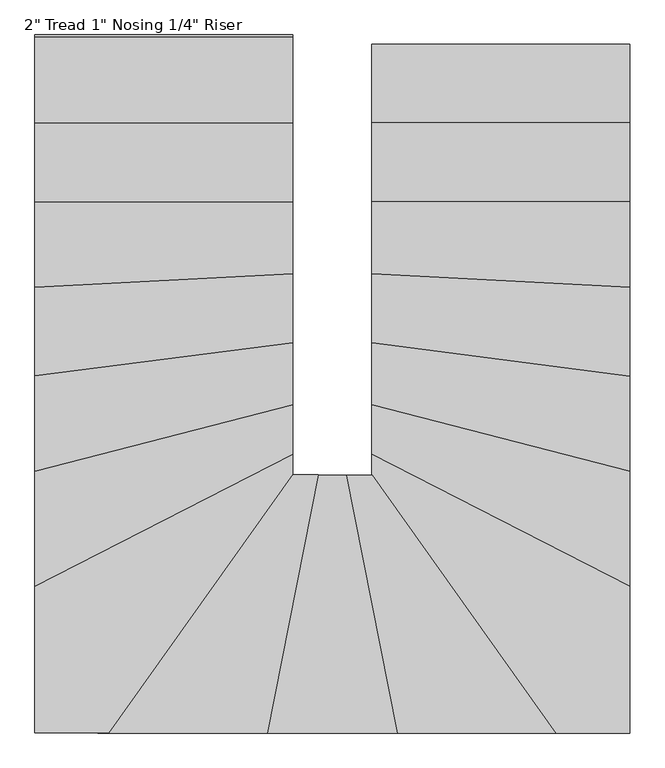
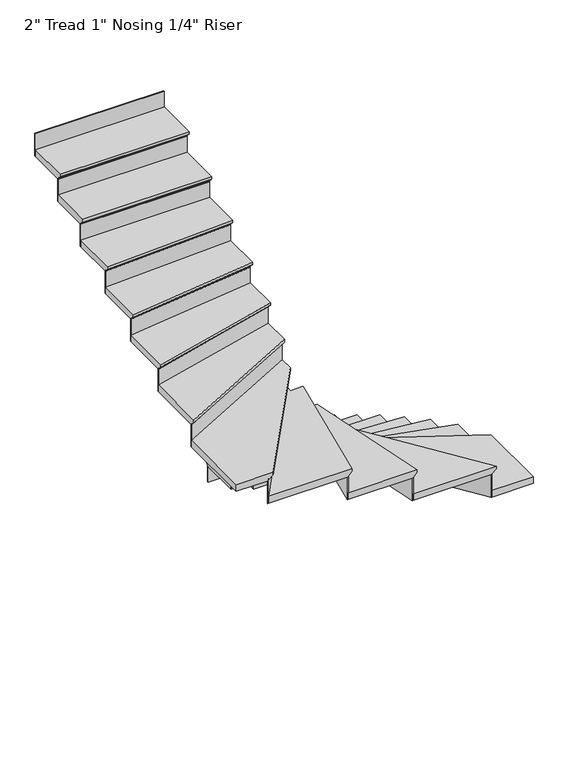
"""IFC4 building model written with IfcOpenShell, lengths in millimetres: stair flight geometry."""

from ifc_helpers import new_model, si_unit, origin, place, context, project, spatial, faceted_brep, source, transform, mapped, element, save


def stair_flight_35bc4011(model_context):
    return source(origin(), model_context, "Body", "Brep", [
        faceted_brep([(-1468.3479637, 880.742092, 150.2833333), (-1468.3479637, 880.742092, 169.3333333), (-553.9479637, 880.742092, 169.3333333), (-553.9479637, 880.742092, 150.2833333), (-1468.3479637, 855.342092, 124.8833333), (-553.9479637, 855.342092, 124.8833333), (-1468.3479637, 575.942092, 169.3333333), (-553.9479637, 575.942092, 169.3333333), (-553.9479637, 855.342092, 118.5333333), (-553.9479637, 575.942092, 118.5333333), (-1468.3479637, 575.942092, 118.5333333), (-1468.3479637, 855.342092, 118.5333333)], [[[0, 1, 2, 3]], [[4, 0, 3, 5]], [[2, 1, 6, 7]], [[8, 9, 10, 11]], [[2, 7, 9, 8, 5, 3]], [[8, 11, 4, 5]], [[6, 1, 0, 4, 11, 10]], [[7, 6, 10, 9]]]),
        faceted_brep([(-1468.3479637, 855.342092, 118.5333333), (-1468.3479637, 855.342092, 0.0), (-1468.3479637, 848.992092, 0.0), (-1468.3479637, 848.992092, 118.5333333), (-553.9479637, 855.342092, 118.5333333), (-553.9479637, 848.992092, 118.5333333), (-553.9479637, 848.992092, 0.0), (-553.9479637, 855.342092, 0.0)], [[[0, 1, 2, 3]], [[4, 5, 6, 7]], [[1, 0, 4, 7]], [[2, 1, 7, 6]], [[3, 2, 6, 5]], [[0, 3, 5, 4]]]),
        faceted_brep([(-1468.3479637, 575.942092, 287.8666667), (-1468.3479637, 575.942092, 118.5333333), (-1468.3479637, 569.592092, 118.5333333), (-1468.3479637, 569.592092, 287.8666667), (-553.9479637, 575.942092, 287.8666667), (-553.9479637, 569.592092, 287.8666667), (-553.9479637, 569.592092, 118.5333333), (-553.9479637, 575.942092, 118.5333333)], [[[0, 1, 2, 3]], [[4, 5, 6, 7]], [[1, 0, 4, 7]], [[2, 1, 7, 6]], [[3, 2, 6, 5]], [[0, 3, 5, 4]]]),
        faceted_brep([(-553.9479637, 601.342092, 338.6666667), (-1468.3479637, 601.342092, 338.6666667), (-1468.3479637, 296.542092, 338.6666667), (-553.9479637, 296.542092, 338.6666667), (-553.9479637, 575.942092, 287.8666667), (-553.9479637, 296.542092, 287.8666667), (-1468.3479637, 296.542092, 287.8666667), (-1468.3479637, 575.942092, 287.8666667), (-553.9479637, 575.942092, 294.2166667), (-553.9479637, 601.342092, 319.6166667), (-1468.3479637, 575.942092, 294.2166667), (-1468.3479637, 601.342092, 319.6166667)], [[[0, 1, 2, 3]], [[4, 5, 6, 7]], [[0, 3, 5, 4, 8, 9]], [[4, 7, 10, 8]], [[2, 1, 11, 10, 7, 6]], [[3, 2, 6, 5]], [[11, 1, 0, 9]], [[10, 11, 9, 8]]]),
        faceted_brep([(-1468.3479637, 296.542092, 457.2), (-1468.3479637, 296.542092, 287.8666667), (-1468.3479637, 290.192092, 287.8666667), (-1468.3479637, 290.192092, 457.2), (-553.9479637, 296.542092, 457.2), (-553.9479637, 290.192092, 457.2), (-553.9479637, 290.192092, 287.8666667), (-553.9479637, 296.542092, 287.8666667)], [[[0, 1, 2, 3]], [[4, 5, 6, 7]], [[1, 0, 4, 7]], [[2, 1, 7, 6]], [[3, 2, 6, 5]], [[0, 3, 5, 4]]]),
        faceted_brep([(-553.9479637, 321.942092, 508.0), (-1468.3479637, 321.942092, 508.0), (-1468.3479637, 40.8749305, 508.0), (-553.9479637, -6.6593399, 508.0), (-553.9479637, 296.542092, 457.2), (-553.9479637, -6.6593399, 457.2), (-1468.3479637, 40.8749305, 457.2), (-1468.3479637, 296.542092, 457.2), (-553.9479637, 296.542092, 463.55), (-553.9479637, 321.942092, 488.95), (-1468.3479637, 296.542092, 463.55), (-1468.3479637, 321.942092, 488.95)], [[[0, 1, 2, 3]], [[4, 5, 6, 7]], [[0, 3, 5, 4, 8, 9]], [[4, 7, 10, 8]], [[2, 1, 11, 10, 7, 6]], [[3, 2, 6, 5]], [[11, 1, 0, 9]], [[10, 11, 9, 8]]]),
        faceted_brep([(-1468.3479637, 40.8749305, 626.5333333), (-1468.3479637, 40.8749305, 457.2), (-1468.3479637, 34.5163563, 457.2), (-1468.3479637, 34.5163563, 626.5333333), (-553.9479637, -6.6593399, 626.5333333), (-553.9479637, -13.0179141, 626.5333333), (-553.9479637, -13.0179141, 457.2), (-553.9479637, -6.6593399, 457.2)], [[[0, 1, 2, 3]], [[4, 5, 6, 7]], [[1, 0, 4, 7]], [[2, 1, 7, 6]], [[3, 2, 6, 5]], [[0, 3, 5, 4]]]),
        faceted_brep([(-553.9479637, 18.7749568, 677.3333333), (-1468.3479637, 66.3092272, 677.3333333), (-1468.3479637, -203.2917693, 677.3333333), (-553.9479637, -321.647821, 677.3333333), (-553.9479637, -6.6593399, 626.5333333), (-553.9479637, -321.647821, 626.5333333), (-1468.3479637, -203.2917693, 626.5333333), (-1468.3479637, 40.8749305, 626.5333333), (-553.9479637, -6.6593399, 632.8833333), (-553.9479637, 18.7749568, 658.2833333), (-1468.3479637, 40.8749305, 632.8833333), (-1468.3479637, 66.3092272, 658.2833333)], [[[0, 1, 2, 3]], [[4, 5, 6, 7]], [[0, 3, 5, 4, 8, 9]], [[4, 7, 10, 8]], [[2, 1, 11, 10, 7, 6]], [[3, 2, 6, 5]], [[11, 1, 0, 9]], [[10, 11, 9, 8]]]),
        faceted_brep([(-1468.3479637, -203.2917693, 795.8666667), (-1468.3479637, -203.2917693, 626.5333333), (-1468.3479637, -209.6947411, 626.5333333), (-1468.3479637, -209.6947411, 795.8666667), (-553.9479637, -321.647821, 795.8666667), (-553.9479637, -328.0507928, 795.8666667), (-553.9479637, -328.0507928, 626.5333333), (-553.9479637, -321.647821, 626.5333333)], [[[0, 1, 2, 3]], [[4, 5, 6, 7]], [[1, 0, 4, 7]], [[2, 1, 7, 6]], [[3, 2, 6, 5]], [[0, 3, 5, 4]]]),
        faceted_brep([(-553.9479637, -296.0359339, 846.6666667), (-1468.3479637, -177.6798822, 846.6666667), (-1468.3479637, -424.9189918, 846.6666667), (-553.9479637, -660.0494392, 846.6666667), (-553.9479637, -321.647821, 795.8666667), (-553.9479637, -660.0494392, 795.8666667), (-1468.3479637, -424.9189918, 795.8666667), (-1468.3479637, -203.2917693, 795.8666667), (-553.9479637, -321.647821, 802.2166667), (-553.9479637, -296.0359339, 827.6166667), (-1468.3479637, -203.2917693, 802.2166667), (-1468.3479637, -177.6798822, 827.6166667)], [[[0, 1, 2, 3]], [[4, 5, 6, 7]], [[0, 3, 5, 4, 8, 9]], [[4, 7, 10, 8]], [[2, 1, 11, 10, 7, 6]], [[3, 2, 6, 5]], [[11, 1, 0, 9]], [[10, 11, 9, 8]]]),
        faceted_brep([(-1468.3479637, -424.9189918, 965.2), (-1468.3479637, -424.9189918, 795.8666667), (-1468.3479637, -431.4755687, 795.8666667), (-1468.3479637, -431.4755687, 965.2), (-553.9479637, -660.0494392, 965.2), (-553.9479637, -666.6060161, 965.2), (-553.9479637, -666.6060161, 795.8666667), (-553.9479637, -660.0494392, 795.8666667)], [[[0, 1, 2, 3]], [[4, 5, 6, 7]], [[1, 0, 4, 7]], [[2, 1, 7, 6]], [[3, 2, 6, 5]], [[0, 3, 5, 4]]]),
        faceted_brep([(-553.9479637, -633.8231317, 1016.0), (-1468.3479637, -398.6926843, 1016.0), (-1468.3479637, -601.2656279, 1016.0), (-553.9479637, -1070.0902492, 1016.0), (-553.9479637, -660.0494392, 965.2), (-553.9479637, -1070.0902492, 965.2), (-1468.3479637, -601.2656279, 965.2), (-1468.3479637, -424.9189918, 965.2), (-553.9479637, -660.0494392, 971.55), (-553.9479637, -633.8231317, 996.95), (-1468.3479637, -424.9189918, 971.55), (-1468.3479637, -398.6926843, 996.95)], [[[0, 1, 2, 3]], [[4, 5, 6, 7]], [[0, 3, 5, 4, 8, 9]], [[4, 7, 10, 8]], [[2, 1, 11, 10, 7, 6]], [[3, 2, 6, 5]], [[11, 1, 0, 9]], [[10, 11, 9, 8]]]),
        faceted_brep([(-1468.3479637, -601.2656279, 1134.5333333), (-1468.3479637, -601.2656279, 965.2), (-1468.3479637, -608.401611, 965.2), (-1468.3479637, -608.401611, 1134.5333333), (-553.9479637, -1070.0902492, 1134.5333333), (-553.9479637, -1077.2262323, 1134.5333333), (-553.9479637, -1077.2262323, 965.2), (-553.9479637, -1070.0902492, 965.2)], [[[0, 1, 2, 3]], [[4, 5, 6, 7]], [[1, 0, 4, 7]], [[2, 1, 7, 6]], [[3, 2, 6, 5]], [[0, 3, 5, 4]]]),
        faceted_brep([(-847.6290974, -1561.3895999, 1185.3333333), (-553.9479637, -1561.3895999, 1185.3333333), (-553.9479637, -1041.5463167, 1185.3333333), (-1468.3479637, -572.7216953, 1185.3333333), (-1468.3479637, -646.9895999, 1185.3333333), (-1497.9030465, -646.9895999, 1185.3333333), (-553.9479637, -1561.3895999, 1134.5333333), (-847.6290974, -1561.3895999, 1134.5333333), (-1497.9030465, -646.9895999, 1134.5333333), (-1468.3479637, -646.9895999, 1134.5333333), (-1468.3479637, -601.2656279, 1134.5333333), (-553.9479637, -1070.0902492, 1134.5333333), (-553.9479637, -1070.0902492, 1140.8833333), (-553.9479637, -1041.5463167, 1166.2833333), (-1468.3479637, -601.2656279, 1140.8833333), (-1468.3479637, -572.7216953, 1166.2833333)], [[[0, 1, 2, 3, 4, 5]], [[6, 7, 8, 9, 10, 11]], [[1, 0, 7, 6]], [[2, 1, 6, 11, 12, 13]], [[11, 10, 14, 12]], [[4, 3, 15, 14, 10, 9]], [[5, 4, 9, 8]], [[0, 5, 8, 7]], [[15, 3, 2, 13]], [[14, 15, 13, 12]]]),
        faceted_brep([(-1497.9030465, -646.9895999, 1303.8666667), (-1497.9030465, -646.9895999, 1134.5333333), (-1505.6950213, -646.9895999, 1134.5333333), (-1505.6950213, -646.9895999, 1303.8666667), (-847.6290974, -1561.3895999, 1303.8666667), (-855.4210722, -1561.3895999, 1303.8666667), (-855.4210722, -1561.3895999, 1134.5333333), (-847.6290974, -1561.3895999, 1134.5333333)], [[[0, 1, 2, 3]], [[4, 5, 6, 7]], [[1, 0, 4, 7]], [[2, 1, 7, 6]], [[3, 2, 6, 5]], [[0, 3, 5, 4]]]),
        faceted_brep([(-816.4611982, -1561.3895999, 1354.6666667), (-1466.7351474, -646.9895999, 1354.6666667), (-1584.3571336, -646.9895999, 1354.6666667), (-1404.1162773, -1561.3895999, 1354.6666667), (-847.6290974, -1561.3895999, 1303.8666667), (-1404.1162773, -1561.3895999, 1303.8666667), (-1584.3571336, -646.9895999, 1303.8666667), (-1497.9030465, -646.9895999, 1303.8666667), (-847.6290974, -1561.3895999, 1310.2166667), (-816.4611982, -1561.3895999, 1335.6166667), (-1497.9030465, -646.9895999, 1310.2166667), (-1466.7351474, -646.9895999, 1335.6166667)], [[[0, 1, 2, 3]], [[4, 5, 6, 7]], [[0, 3, 5, 4, 8, 9]], [[4, 7, 10, 8]], [[2, 1, 11, 10, 7, 6]], [[3, 2, 6, 5]], [[11, 1, 0, 9]], [[10, 11, 9, 8]]]),
        faceted_brep([(-1584.3571336, -646.9895999, 1473.2), (-1584.3571336, -646.9895999, 1303.8666667), (-1590.829319, -646.9895999, 1303.8666667), (-1590.829319, -646.9895999, 1473.2), (-1404.1162773, -1561.3895999, 1473.2), (-1410.5884627, -1561.3895999, 1473.2), (-1410.5884627, -1561.3895999, 1303.8666667), (-1404.1162773, -1561.3895999, 1303.8666667)], [[[0, 1, 2, 3]], [[4, 5, 6, 7]], [[1, 0, 4, 7]], [[2, 1, 7, 6]], [[3, 2, 6, 5]], [[0, 3, 5, 4]]]),
        faceted_brep([(-1378.2275355, -1561.3895999, 1524.0), (-1558.4683919, -646.9895999, 1524.0), (-1683.5162773, -646.9895999, 1524.0), (-1863.7571336, -1561.3895999, 1524.0), (-1404.1162773, -1561.3895999, 1473.2), (-1863.7571336, -1561.3895999, 1473.2), (-1683.5162773, -646.9895999, 1473.2), (-1584.3571336, -646.9895999, 1473.2), (-1404.1162773, -1561.3895999, 1479.55), (-1378.2275355, -1561.3895999, 1504.95), (-1584.3571336, -646.9895999, 1479.55), (-1558.4683919, -646.9895999, 1504.95)], [[[0, 1, 2, 3]], [[4, 5, 6, 7]], [[0, 3, 5, 4, 8, 9]], [[4, 7, 10, 8]], [[2, 1, 11, 10, 7, 6]], [[3, 2, 6, 5]], [[11, 1, 0, 9]], [[10, 11, 9, 8]]]),
        faceted_brep([(-1683.5162773, -646.9895999, 1642.5333333), (-1683.5162773, -646.9895999, 1473.2), (-1689.9884627, -646.9895999, 1473.2), (-1689.9884627, -646.9895999, 1642.5333333), (-1863.7571336, -1561.3895999, 1642.5333333), (-1870.229319, -1561.3895999, 1642.5333333), (-1870.229319, -1561.3895999, 1473.2), (-1863.7571336, -1561.3895999, 1473.2)], [[[0, 1, 2, 3]], [[4, 5, 6, 7]], [[1, 0, 4, 7]], [[2, 1, 7, 6]], [[3, 2, 6, 5]], [[0, 3, 5, 4]]]),
        faceted_brep([(-1837.8683919, -1561.3895999, 1693.3333333), (-1657.6275355, -646.9895999, 1693.3333333), (-1747.7479637, -646.9895999, 1693.3333333), (-1747.7479637, -600.8941254, 1693.3333333), (-2430.8026283, -1561.3895999, 1693.3333333), (-1863.7571336, -1561.3895999, 1642.5333333), (-2430.8026283, -1561.3895999, 1642.5333333), (-1747.7479637, -600.8941254, 1642.5333333), (-1747.7479637, -646.9895999, 1642.5333333), (-1683.5162773, -646.9895999, 1642.5333333), (-1863.7571336, -1561.3895999, 1648.8833333), (-1837.8683919, -1561.3895999, 1674.2833333), (-1683.5162773, -646.9895999, 1648.8833333), (-1657.6275355, -646.9895999, 1674.2833333)], [[[0, 1, 2, 3, 4]], [[5, 6, 7, 8, 9]], [[0, 4, 6, 5, 10, 11]], [[5, 9, 12, 10]], [[2, 1, 13, 12, 9, 8]], [[3, 2, 8, 7]], [[4, 3, 7, 6]], [[13, 1, 0, 11]], [[12, 13, 11, 10]]]),
        faceted_brep([(-1747.7479637, -600.8941254, 1811.8666667), (-1747.7479637, -600.8941254, 1642.5333333), (-1747.7479637, -589.9372329, 1642.5333333), (-1747.7479637, -589.9372329, 1811.8666667), (-2430.8026283, -1561.3895999, 1811.8666667), (-2438.5946031, -1561.3895999, 1811.8666667), (-2438.5946031, -1561.3895999, 1642.5333333), (-2430.8026283, -1561.3895999, 1642.5333333)], [[[0, 1, 2, 3]], [[4, 5, 6, 7]], [[1, 0, 4, 7]], [[2, 1, 7, 6]], [[3, 2, 6, 5]], [[0, 3, 5, 4]]]),
        faceted_brep([(-2662.1479637, -1013.0023841, 1862.6666667), (-2662.1479637, -1561.3895999, 1862.6666667), (-2399.6347292, -1561.3895999, 1862.6666667), (-1747.7479637, -644.7216953, 1862.6666667), (-1747.7479637, -544.1777628, 1862.6666667), (-2662.1479637, -1561.3895999, 1811.8666667), (-2662.1479637, -1013.0023841, 1811.8666667), (-1747.7479637, -544.1777628, 1811.8666667), (-1747.7479637, -600.8941254, 1811.8666667), (-2430.8026283, -1561.3895999, 1811.8666667), (-2430.8026283, -1561.3895999, 1818.2166667), (-2399.6347292, -1561.3895999, 1843.6166667), (-1747.7479637, -600.8941254, 1818.2166667), (-1747.7479637, -644.7216953, 1843.6166667)], [[[0, 1, 2, 3, 4]], [[5, 6, 7, 8, 9]], [[1, 0, 6, 5]], [[2, 1, 5, 9, 10, 11]], [[9, 8, 12, 10]], [[4, 3, 13, 12, 8, 7]], [[0, 4, 7, 6]], [[13, 3, 2, 11]], [[12, 13, 11, 10]]]),
        faceted_brep([(-1747.7479637, -544.1777628, 1981.2), (-1747.7479637, -544.1777628, 1811.8666667), (-1747.7479637, -537.0417797, 1811.8666667), (-1747.7479637, -537.0417797, 1981.2), (-2662.1479637, -1013.0023841, 1981.2), (-2662.1479637, -1005.866401, 1981.2), (-2662.1479637, -1005.866401, 1811.8666667), (-2662.1479637, -1013.0023841, 1811.8666667)], [[[0, 1, 2, 3]], [[4, 5, 6, 7]], [[1, 0, 4, 7]], [[2, 1, 7, 6]], [[3, 2, 6, 5]], [[0, 3, 5, 4]]]),
        faceted_brep([(-2662.1479637, -1041.5463167, 2032.0), (-1747.7479637, -572.7216953, 2032.0), (-1747.7479637, -372.4663769, 2032.0), (-2662.1479637, -607.5968243, 2032.0), (-2662.1479637, -1013.0023841, 1981.2), (-2662.1479637, -607.5968243, 1981.2), (-1747.7479637, -372.4663769, 1981.2), (-1747.7479637, -544.1777628, 1981.2), (-2662.1479637, -1013.0023841, 1987.55), (-2662.1479637, -1041.5463167, 2012.95), (-1747.7479637, -544.1777628, 1987.55), (-1747.7479637, -572.7216953, 2012.95)], [[[0, 1, 2, 3]], [[4, 5, 6, 7]], [[0, 3, 5, 4, 8, 9]], [[4, 7, 10, 8]], [[2, 1, 11, 10, 7, 6]], [[3, 2, 6, 5]], [[11, 1, 0, 9]], [[10, 11, 9, 8]]]),
        faceted_brep([(-1747.7479637, -372.4663769, 2150.5333333), (-1747.7479637, -372.4663769, 1981.2), (-1747.7479637, -365.9098, 1981.2), (-1747.7479637, -365.9098, 2150.5333333), (-2662.1479637, -607.5968243, 2150.5333333), (-2662.1479637, -601.0402474, 2150.5333333), (-2662.1479637, -601.0402474, 1981.2), (-2662.1479637, -607.5968243, 1981.2)], [[[0, 1, 2, 3]], [[4, 5, 6, 7]], [[1, 0, 4, 7]], [[2, 1, 7, 6]], [[3, 2, 6, 5]], [[0, 3, 5, 4]]]),
        faceted_brep([(-2662.1479637, -633.8231317, 2201.3333333), (-1747.7479637, -398.6926843, 2201.3333333), (-1747.7479637, -152.0679951, 2201.3333333), (-2662.1479637, -270.4240468, 2201.3333333), (-2662.1479637, -607.5968243, 2150.5333333), (-2662.1479637, -270.4240468, 2150.5333333), (-1747.7479637, -152.0679951, 2150.5333333), (-1747.7479637, -372.4663769, 2150.5333333), (-2662.1479637, -607.5968243, 2156.8833333), (-2662.1479637, -633.8231317, 2182.2833333), (-1747.7479637, -372.4663769, 2156.8833333), (-1747.7479637, -398.6926843, 2182.2833333)], [[[0, 1, 2, 3]], [[4, 5, 6, 7]], [[0, 3, 5, 4, 8, 9]], [[4, 7, 10, 8]], [[2, 1, 11, 10, 7, 6]], [[3, 2, 6, 5]], [[11, 1, 0, 9]], [[10, 11, 9, 8]]]),
        faceted_brep([(-1747.7479637, -152.0679951, 2319.8666667), (-1747.7479637, -152.0679951, 2150.5333333), (-1747.7479637, -145.6650233, 2150.5333333), (-1747.7479637, -145.6650233, 2319.8666667), (-2662.1479637, -270.4240468, 2319.8666667), (-2662.1479637, -264.021075, 2319.8666667), (-2662.1479637, -264.021075, 2150.5333333), (-2662.1479637, -270.4240468, 2150.5333333)], [[[0, 1, 2, 3]], [[4, 5, 6, 7]], [[1, 0, 4, 7]], [[2, 1, 7, 6]], [[3, 2, 6, 5]], [[0, 3, 5, 4]]]),
        faceted_brep([(-2662.1479637, -296.0359339, 2370.6666667), (-1747.7479637, -177.6798822, 2370.6666667), (-1747.7479637, 91.7435238, 2370.6666667), (-2662.1479637, 44.2092534, 2370.6666667), (-2662.1479637, -270.4240468, 2319.8666667), (-2662.1479637, 44.2092534, 2319.8666667), (-1747.7479637, 91.7435238, 2319.8666667), (-1747.7479637, -152.0679951, 2319.8666667), (-2662.1479637, -270.4240468, 2326.2166667), (-2662.1479637, -296.0359339, 2351.6166667), (-1747.7479637, -152.0679951, 2326.2166667), (-1747.7479637, -177.6798822, 2351.6166667)], [[[0, 1, 2, 3]], [[4, 5, 6, 7]], [[0, 3, 5, 4, 8, 9]], [[4, 7, 10, 8]], [[2, 1, 11, 10, 7, 6]], [[3, 2, 6, 5]], [[11, 1, 0, 9]], [[10, 11, 9, 8]]]),
        faceted_brep([(-1747.7479637, 91.7435238, 2489.2), (-1747.7479637, 91.7435238, 2319.8666667), (-1747.7479637, 98.102098, 2319.8666667), (-1747.7479637, 98.102098, 2489.2), (-2662.1479637, 44.2092534, 2489.2), (-2662.1479637, 50.5678276, 2489.2), (-2662.1479637, 50.5678276, 2319.8666667), (-2662.1479637, 44.2092534, 2319.8666667)], [[[0, 1, 2, 3]], [[4, 5, 6, 7]], [[1, 0, 4, 7]], [[2, 1, 7, 6]], [[3, 2, 6, 5]], [[0, 3, 5, 4]]]),
        faceted_brep([(-2662.1479637, 18.7749568, 2540.0), (-1747.7479637, 66.3092272, 2540.0), (-1747.7479637, 347.342092, 2540.0), (-2662.1479637, 347.342092, 2540.0), (-2662.1479637, 44.2092534, 2489.2), (-2662.1479637, 347.342092, 2489.2), (-1747.7479637, 347.342092, 2489.2), (-1747.7479637, 91.7435238, 2489.2), (-2662.1479637, 44.2092534, 2495.55), (-2662.1479637, 18.7749568, 2520.95), (-1747.7479637, 91.7435238, 2495.55), (-1747.7479637, 66.3092272, 2520.95)], [[[0, 1, 2, 3]], [[4, 5, 6, 7]], [[0, 3, 5, 4, 8, 9]], [[4, 7, 10, 8]], [[2, 1, 11, 10, 7, 6]], [[3, 2, 6, 5]], [[11, 1, 0, 9]], [[10, 11, 9, 8]]]),
        faceted_brep([(-1747.7479637, 347.342092, 2658.5333333), (-1747.7479637, 347.342092, 2489.2), (-1747.7479637, 353.692092, 2489.2), (-1747.7479637, 353.692092, 2658.5333333), (-2662.1479637, 347.342092, 2658.5333333), (-2662.1479637, 353.692092, 2658.5333333), (-2662.1479637, 353.692092, 2489.2), (-2662.1479637, 347.342092, 2489.2)], [[[0, 1, 2, 3]], [[4, 5, 6, 7]], [[1, 0, 4, 7]], [[2, 1, 7, 6]], [[3, 2, 6, 5]], [[0, 3, 5, 4]]]),
        faceted_brep([(-2662.1479637, 321.942092, 2709.3333333), (-1747.7479637, 321.942092, 2709.3333333), (-1747.7479637, 626.742092, 2709.3333333), (-2662.1479637, 626.742092, 2709.3333333), (-2662.1479637, 347.342092, 2658.5333333), (-2662.1479637, 626.742092, 2658.5333333), (-1747.7479637, 626.742092, 2658.5333333), (-1747.7479637, 347.342092, 2658.5333333), (-2662.1479637, 347.342092, 2664.8833333), (-2662.1479637, 321.942092, 2690.2833333), (-1747.7479637, 347.342092, 2664.8833333), (-1747.7479637, 321.942092, 2690.2833333)], [[[0, 1, 2, 3]], [[4, 5, 6, 7]], [[0, 3, 5, 4, 8, 9]], [[4, 7, 10, 8]], [[2, 1, 11, 10, 7, 6]], [[3, 2, 6, 5]], [[11, 1, 0, 9]], [[10, 11, 9, 8]]]),
        faceted_brep([(-1747.7479637, 626.742092, 2827.8666667), (-1747.7479637, 626.742092, 2658.5333333), (-1747.7479637, 633.092092, 2658.5333333), (-1747.7479637, 633.092092, 2827.8666667), (-2662.1479637, 626.742092, 2827.8666667), (-2662.1479637, 633.092092, 2827.8666667), (-2662.1479637, 633.092092, 2658.5333333), (-2662.1479637, 626.742092, 2658.5333333)], [[[0, 1, 2, 3]], [[4, 5, 6, 7]], [[1, 0, 4, 7]], [[2, 1, 7, 6]], [[3, 2, 6, 5]], [[0, 3, 5, 4]]]),
        faceted_brep([(-1747.7479637, 906.142092, 2997.2), (-1747.7479637, 906.142092, 2827.8666667), (-1747.7479637, 912.492092, 2827.8666667), (-1747.7479637, 912.492092, 2997.2), (-2662.1479637, 906.142092, 2997.2), (-2662.1479637, 912.492092, 2997.2), (-2662.1479637, 912.492092, 2827.8666667), (-2662.1479637, 906.142092, 2827.8666667)], [[[0, 1, 2, 3]], [[4, 5, 6, 7]], [[1, 0, 4, 7]], [[2, 1, 7, 6]], [[3, 2, 6, 5]], [[0, 3, 5, 4]]]),
        faceted_brep([(-2662.1479637, 601.342092, 2878.6666667), (-1747.7479637, 601.342092, 2878.6666667), (-1747.7479637, 906.142092, 2878.6666667), (-2662.1479637, 906.142092, 2878.6666667), (-2662.1479637, 626.742092, 2827.8666667), (-2662.1479637, 906.142092, 2827.8666667), (-1747.7479637, 906.142092, 2827.8666667), (-1747.7479637, 626.742092, 2827.8666667), (-2662.1479637, 626.742092, 2834.2166667), (-2662.1479637, 601.342092, 2859.6166667), (-1747.7479637, 626.742092, 2834.2166667), (-1747.7479637, 601.342092, 2859.6166667)], [[[0, 1, 2, 3]], [[4, 5, 6, 7]], [[0, 3, 5, 4, 8, 9]], [[4, 7, 10, 8]], [[2, 1, 11, 10, 7, 6]], [[3, 2, 6, 5]], [[11, 1, 0, 9]], [[10, 11, 9, 8]]]),
    ])


if __name__ == "__main__":
    model = new_model("IFC4")
    model_context = context("Model", 3, world=origin())
    ifc_project = project(units=[si_unit("LENGTHUNIT", "METRE", prefix="MILLI")], contexts=[model_context])
    site = spatial("IfcSite", under=ifc_project)
    building = spatial("IfcBuilding", under=site)
    placement = place(None, origin())
    stair_flight_shape = stair_flight_35bc4011(model_context)
    element("IfcStairFlight", 1, ObjectType="2\" Tread 1\" Nosing 1/4\" Riser", at=placement, inside=building, context=model_context, shape_type="MappedRepresentation", body=[
        mapped(stair_flight_shape, transform((0.0, 0.0, 0.0), x_axis=(1.0, 0.0, 0.0), y_axis=(0.0, 1.0, 0.0), z_axis=(0.0, 0.0, 1.0))),
    ])
    save(model, "model.ifc")
